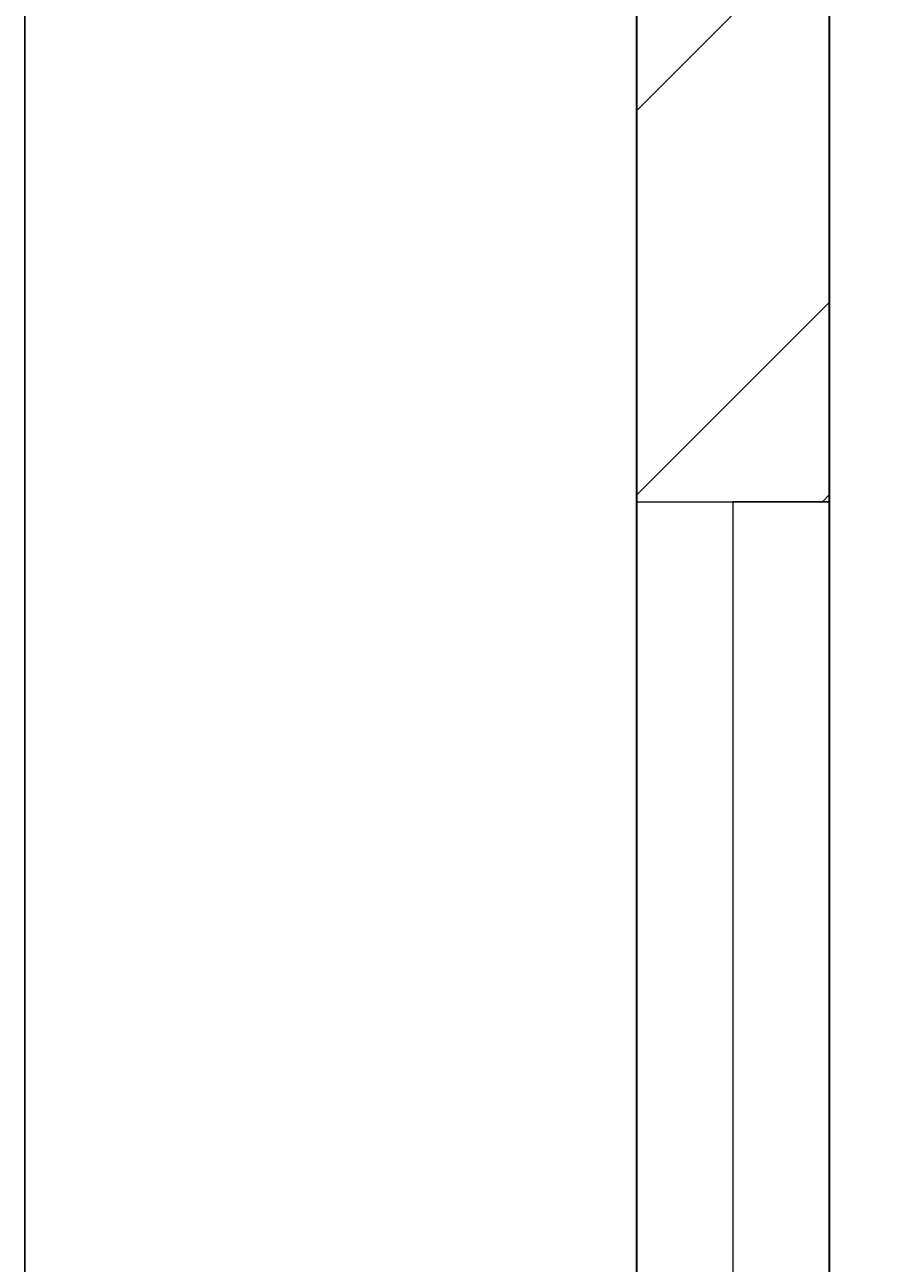
# Model space of a CAD drawing. Units: inches. Extents: x 1962 to 2771, y 1245 to 2660.
# Tile 47 of 114: x 2072 to 2092, y 2122 to 2151. Entities that reach past the tile are written whole.
import ezdxf

# ---------------------------------------------------------------- set-up
doc = ezdxf.new("R2010")
doc.units = ezdxf.units.IN
for name, color, linetype, lineweight in [('A-ANNO-DIMS', 2, 'Continuous', 18), ('A-GLAZ', 4, 'Continuous', 18), ('A-WALL', 7, 'Continuous', 35), ('A-WALL-PATT', 252, 'Continuous', 13)]:
    doc.layers.add(name, color=color, linetype=linetype, lineweight=lineweight)
doc.styles.get("Standard").update_dxf_attribs({"font": 'arial.ttf'})
doc.dimstyles.get("Standard").update_dxf_attribs({"dimtxt": 0.18, "dimasz": 0.18, "dimexe": 0.18, "dimexo": 0.0625, "dimgap": 0.09, "dimtad": 0, "dimtih": 1, "dimtoh": 1, "dimdec": 4, "dimzin": 0, "dimdsep": 46, "dimtxsty": 'Standard', "dimcen": 0.09, "dimadec": 0, "dimazin": 0, "dimtfac": 1, "dimtdec": 4, "dimtofl": 0, "dimtmove": 0, "dimatfit": 3, "dimfxl": 1, "dimtolj": 1, "dimtzin": 0, "dimarcsym": 0})

# ---------------------------------------------------------------- blocks, each defined once
blk = doc.blocks.new('WIN-60IN-A')
for p, q in [((0, 60), (4.5, 60)), ((4.5, 60), (2.25, 60)), ((2.25, 60), (2.25, 0))]:
    blk.add_line(p, q)
blk = doc.blocks.new('*D40')
at = {"layer": 'A-ANNO-DIMS', "color": 0, "lineweight": -2, "transparency": 16777216}
for p, q in [((2072.02, 2033.906), (2072.02, 2583.474)), ((2072.2, 2583.294), (2366.02, 2583.294)), ((2660.627, 2583.294), (2366.808, 2583.294)), ((2660.807, 2524.406), (2660.807, 2583.474))]:
    blk.add_line(p, q, dxfattribs=at)
at = {"layer": 'A-ANNO-DIMS', "color": 0, "transparency": 16777216}
for points in [[(2072.2, 2583.324), (2072.2, 2583.264), (2072.02, 2583.294)], [(2660.627, 2583.324), (2660.627, 2583.264), (2660.807, 2583.294)]]:
    blk.add_solid(points, dxfattribs=at)
at = {"layer": 'Defpoints', "color": 0, "transparency": 16777216}
for p in [(2660.807, 2583.294), (2660.807, 2524.344), (2072.02, 2033.844)]:
    blk.add_point(p, dxfattribs=at)
at = {"layer": 'A-ANNO-DIMS', "color": 0, "transparency": 16777216, "insert": (2366.414, 2583.294), "char_height": 0.18, "attachment_point": 5}
blk.add_mtext('\\A1;588.8', dxfattribs=at)
blk = doc.blocks.new('*D43')
at = {"layer": 'A-ANNO-DIMS', "color": 0, "lineweight": -2, "transparency": 16777216}
for p, q in [((2086.245, 2524.344), (2012.89, 2524.344)), ((2013.07, 2524.164), (2013.07, 2279.276)), ((2013.07, 2034.024), (2013.07, 2278.912)), ((2071.958, 2033.844), (2012.89, 2033.844))]:
    blk.add_line(p, q, dxfattribs=at)
at = {"layer": 'A-ANNO-DIMS', "color": 0, "transparency": 16777216}
for points in [[(2013.04, 2524.164), (2013.1, 2524.164), (2013.07, 2524.344)], [(2013.04, 2034.024), (2013.1, 2034.024), (2013.07, 2033.844)]]:
    blk.add_solid(points, dxfattribs=at)
at = {"layer": 'Defpoints', "color": 0, "transparency": 16777216}
for p in [(2086.307, 2524.344), (2013.07, 2033.844), (2072.02, 2033.844)]:
    blk.add_point(p, dxfattribs=at)
at = {"layer": 'A-ANNO-DIMS', "color": 0, "transparency": 16777216, "insert": (2013.07, 2279.094), "char_height": 0.18, "attachment_point": 5}
blk.add_mtext('\\A1;490.5', dxfattribs=at)

msp = doc.modelspace()

# ---------------------------------------------------------------- hatches: boundary and pattern name
at = {"layer": 'A-WALL-PATT'}
h = msp.add_hatch(dxfattribs=at)
h.set_pattern_fill('ANSI32', color=256)
h.paths.add_polyline_path([(2090.8074, 2467.3437), (2141.6481, 2467.3437), (2141.6481, 2469.5937), (2141.6481, 2471.8437), (2086.3074, 2471.8437), (2086.3074, 2422.5333), (2090.8074, 2422.5333)])
h.paths.add_polyline_path([(2282.7664, 2471.8437), (2204.8982, 2471.8437), (2204.8982, 2467.3437), (2234.8074, 2467.3437), (2234.8074, 2311.3437), (2228.7492, 2311.3437), (2228.7492, 2306.8437), (2234.8074, 2306.8437), (2331.9227, 2306.8437), (2331.9227, 2309.0937), (2331.9227, 2311.3437), (2239.3074, 2311.3437), (2239.3074, 2467.3437), (2282.7664, 2467.3437), (2282.7664, 2469.5937)])
h.paths.add_polyline_path([(2471.4531, 2519.8437), (2552.011, 2519.8437), (2564.3996, 2519.8437), (2564.3996, 2511.1389), (2568.8996, 2511.1389), (2568.8996, 2524.3437), (2466.9531, 2524.3437), (2466.9531, 2471.8437), (2450.0749, 2471.8437), (2446.4672, 2471.8437), (2446.4672, 2467.3437), (2450.0749, 2467.3437), (2475.9988, 2467.3437), (2475.9988, 2469.5937), (2475.9988, 2471.8437), (2471.4531, 2471.8437)])
h.paths.add_polyline_path([(2575.2231, 2469.5937), (2575.2231, 2471.8437), (2568.8996, 2471.8437), (2568.8996, 2487.1389), (2564.3996, 2487.1389), (2564.3996, 2471.8437), (2556.511, 2471.8437), (2499.2904, 2471.8437), (2499.2904, 2467.3437), (2507.8074, 2467.3437), (2507.8074, 2311.3437), (2414.863, 2311.3437), (2414.863, 2306.8437), (2512.3074, 2306.8437), (2517.0114, 2306.8437), (2517.0114, 2309.0937), (2517.0114, 2311.3437), (2512.3074, 2311.3437), (2512.3074, 2467.3437), (2575.2231, 2467.3437)])
h.paths.add_polyline_path([(2660.8074, 2471.8437), (2600.9602, 2471.8437), (2600.9602, 2467.3437), (2656.3074, 2467.3437), (2656.3074, 2432.5704), (2660.8074, 2432.5704)])
h.paths.add_polyline_path([(2660.8074, 2372.5704), (2656.3074, 2372.5704), (2656.3074, 2311.3437), (2600.276, 2311.3437), (2600.276, 2309.0937), (2600.276, 2306.8437), (2656.3074, 2306.8437), (2656.3074, 2296.2593), (2660.8074, 2296.2593)])
h.paths.add_polyline_path([(2572.3074, 2306.8437), (2577.1385, 2306.8437), (2577.1385, 2311.3437), (2551.082, 2311.3437), (2551.082, 2306.8437), (2567.8074, 2306.8437), (2567.8074, 2258.8437), (2540.0574, 2258.8437), (2540.0574, 2256.5937), (2540.0574, 2254.3437), (2567.8074, 2254.3437), (2656.3074, 2254.3437), (2656.3074, 2236.9085), (2660.8074, 2236.9085), (2660.8074, 2272.2593), (2656.3074, 2272.2593), (2656.3074, 2258.8437), (2572.3074, 2258.8437)])
h.paths.add_polyline_path([(2512.3074, 2254.3437), (2518.8716, 2254.3437), (2518.8716, 2256.5937), (2518.8716, 2258.8437), (2507.8074, 2258.8437), (2507.8074, 2177.8437), (2567.8074, 2177.8437), (2567.8074, 2172.9628), (2572.3074, 2172.9628), (2572.3074, 2177.8437), (2656.3074, 2177.8437), (2656.3074, 2166.4846), (2660.8074, 2166.4846), (2660.8074, 2200.9085), (2656.3074, 2200.9085), (2656.3074, 2182.3437), (2512.3074, 2182.3437)])
h.paths.add_polyline_path([(2656.3074, 2129.8437), (2572.3074, 2129.8437), (2572.3074, 2150.3044), (2570.0574, 2150.3044), (2567.8074, 2150.3044), (2567.8074, 2129.8437), (2507.8074, 2129.8437), (2507.8074, 2116.3027), (2510.0574, 2116.3027), (2512.3074, 2116.3027), (2512.3074, 2125.3437), (2567.8074, 2125.3437), (2572.3074, 2125.3437), (2656.3074, 2125.3437)])
h.paths.add_polyline_path([(2090.8074, 2362.5333), (2086.3074, 2362.5333), (2086.3074, 2298.6242), (2090.8074, 2298.6242), (2090.8074, 2306.8437), (2174.8074, 2306.8437), (2174.8074, 2286.4178), (2179.3074, 2286.4178), (2179.3074, 2306.8437), (2192.8641, 2306.8437), (2192.8641, 2309.0937), (2192.8641, 2311.3437), (2090.8074, 2311.3437)])
h.paths.add_polyline_path([(2209.156, 2258.8437), (2179.3074, 2258.8437), (2179.3074, 2263.2236), (2177.0574, 2263.2236), (2174.8074, 2263.2236), (2174.8074, 2258.8437), (2090.8074, 2258.8437), (2090.8074, 2274.6242), (2086.3074, 2274.6242), (2086.3074, 2238.2967), (2088.5574, 2238.2967), (2090.8074, 2238.2967), (2090.8074, 2254.3437), (2209.156, 2254.3437)])
h.paths.add_polyline_path([(2090.8074, 2177.8437), (2234.8074, 2177.8437), (2234.8074, 2173.1428), (2239.3074, 2173.1428), (2239.3074, 2258.8437), (2230.8442, 2258.8437), (2230.8442, 2256.5937), (2230.8442, 2254.3437), (2234.8074, 2254.3437), (2234.8074, 2182.3437), (2090.8074, 2182.3437), (2090.8074, 2202.2967), (2086.3074, 2202.2967), (2086.3074, 2140.0389), (2090.8074, 2140.0389)])
h.paths.add_polyline_path([(2090.8074, 2080.0389), (2086.3074, 2080.0389), (2086.3074, 2033.8437), (2090.8074, 2033.8437)], flags=17)
h.paths.add_polyline_path([(2244.9405, 2033.8437), (2239.3074, 2033.8437), (2239.3074, 2142.0665), (2237.2592, 2142.0665), (2234.8074, 2142.0665), (2234.8074, 2033.8437), (2090.8074, 2033.8437), (2076.5204, 2033.8437), (2072.0204, 2033.8437), (2072.0204, 2000.4493), (2076.5204, 2000.4493), (2076.5204, 2029.3437), (2090.8074, 2029.3437), (2244.9405, 2029.3437), (2244.9405, 2031.5937)])
h.paths.add_polyline_path([(2234.8074, 1933.3437), (2076.5204, 1933.3437), (2076.5204, 1952.4493), (2074.2704, 1952.4493), (2072.0204, 1952.4493), (2072.0204, 1933.3437), (2072.0204, 1928.8437), (2234.8074, 1928.8437)])
h.paths.add_polyline_path([(2090.8074, 1928.8437), (2086.3074, 1928.8437), (2086.3074, 1906.5013), (2090.8074, 1906.5013)])
h.paths.add_polyline_path([(2090.8074, 1846.5013), (2086.3074, 1846.5013), (2086.3074, 1769.9917), (2088.5574, 1769.9917), (2090.8074, 1769.9917), (2090.8074, 1780.3437), (2234.8074, 1780.3437), (2234.8074, 1708.3437), (2230.3764, 1708.3437), (2230.3764, 1703.8437), (2239.3074, 1703.8437), (2239.3074, 1792.6669), (2237.0574, 1792.6669), (2234.8074, 1792.6669), (2234.8074, 1784.8437), (2090.8074, 1784.8437)])
h.paths.add_polyline_path([(2239.3074, 1928.8437), (2244.9405, 1928.8437), (2244.9405, 1931.0937), (2244.9405, 1933.3437), (2234.8074, 1933.3437), (2234.8074, 1928.8437), (2234.8074, 1825.5949), (2239.3074, 1825.5949)])
h.paths.add_polyline_path([(2148.0425, 1649.0937), (2148.0425, 1651.3437), (2090.8074, 1651.3437), (2090.8074, 1646.8437), (2148.0425, 1646.8437)], flags=0)
h.paths.add_polyline_path([(2207.5601, 1708.3437), (2090.8074, 1708.3437), (2090.8074, 1703.8437), (2174.8074, 1703.8437), (2174.8074, 1651.3437), (2170.4457, 1651.3437), (2170.4457, 1646.8437), (2195.9924, 1646.8437), (2195.9924, 1649.0937), (2195.9924, 1651.3437), (2179.3074, 1651.3437), (2179.3074, 1703.8437), (2207.5601, 1703.8437), (2207.5601, 1706.0937)])
h.paths.add_polyline_path([(2090.8074, 1733.9917), (2086.3074, 1733.9917), (2086.3074, 1696.1032), (2088.5574, 1696.1032), (2090.8074, 1696.1032)])
h.paths.add_polyline_path([(2090.8074, 1672.1032), (2086.3074, 1672.1032), (2086.3074, 1600.3335), (2090.8074, 1600.3335)])
h.paths.add_polyline_path([(2090.8074, 1540.3335), (2086.3074, 1540.3335), (2086.3074, 1486.3437), (2139.6766, 1486.3437), (2139.6766, 1490.8437), (2090.8074, 1490.8437)])
h.paths.add_polyline_path([(2302.3876, 1490.8437), (2239.3074, 1490.8437), (2239.3074, 1646.8437), (2335.9994, 1646.8437), (2335.9994, 1651.3437), (2229.884, 1651.3437), (2229.884, 1646.8437), (2234.8074, 1646.8437), (2234.8074, 1490.8437), (2202.7103, 1490.8437), (2202.7103, 1488.5937), (2202.7103, 1486.3437), (2275.0699, 1486.3437), (2275.0699, 1475.772), (2279.5699, 1475.772), (2279.5699, 1486.3437), (2302.3876, 1486.3437)])
h.paths.add_polyline_path([(2279.5699, 1451.772), (2275.0699, 1451.772), (2275.0699, 1438.3437), (2174.8074, 1438.3437), (2174.8074, 1486.3437), (2179.7922, 1486.3437), (2179.7922, 1490.8437), (2163.3585, 1490.8437), (2163.3585, 1488.5937), (2163.3585, 1486.3437), (2170.3074, 1486.3437), (2170.3074, 1433.8437), (2279.5699, 1433.8437)])
h.paths.add_polyline_path([(2427.2363, 1490.8437), (2375.8074, 1490.8437), (2375.8074, 1646.8437), (2381.6401, 1646.8437), (2381.6401, 1651.3437), (2365.887, 1651.3437), (2365.887, 1649.0937), (2365.887, 1646.8437), (2371.3074, 1646.8437), (2371.3074, 1490.8437), (2327.5627, 1490.8437), (2327.5627, 1488.5937), (2327.5627, 1486.3437), (2371.3074, 1486.3437), (2371.3074, 1433.8437), (2375.8074, 1433.8437), (2375.8074, 1486.3437), (2427.2363, 1486.3437)])
h.paths.add_polyline_path([(2512.3074, 1646.8437), (2519.4351, 1646.8437), (2519.4351, 1649.0937), (2519.4351, 1651.3437), (2507.8074, 1651.3437), (2416.0063, 1651.3437), (2416.0063, 1649.0937), (2416.0063, 1646.8437), (2507.8074, 1646.8437), (2507.8074, 1490.8437), (2497.0532, 1490.8437), (2497.0532, 1488.5937), (2497.0532, 1486.3437), (2574.9344, 1486.3437), (2574.9344, 1476.0181), (2579.4344, 1476.0181), (2579.4344, 1486.3437), (2584.4872, 1486.3437), (2584.3074, 1490.8437), (2512.3074, 1490.8437)])
h.paths.add_polyline_path([(2470.5091, 1486.3437), (2473.9767, 1486.3437), (2473.9767, 1490.8437), (2449.6605, 1490.8437), (2449.6605, 1488.5937), (2449.6605, 1486.3437), (2466.0091, 1486.3437), (2466.0091, 1433.8437), (2470.5091, 1433.8437), (2579.4344, 1433.8437), (2579.4344, 1452.0181), (2574.9344, 1452.0181), (2574.9344, 1438.3437), (2554.5091, 1438.3437), (2470.5091, 1438.3437)])
h.paths.add_polyline_path([(2656.3074, 1490.8437), (2611.86, 1490.8437), (2611.86, 1486.3437), (2656.3074, 1486.3437)])
h.paths.add_polyline_path([(2660.8074, 1532.7007), (2658.5574, 1532.7007), (2656.3074, 1532.7007), (2656.3074, 1486.3437), (2660.8074, 1486.3437)])
h.paths.add_polyline_path([(2660.8074, 1664.9663), (2656.3074, 1664.9663), (2656.3074, 1651.3437), (2602.2313, 1651.3437), (2602.2313, 1646.8437), (2656.3074, 1646.8437), (2656.3074, 1592.7007), (2660.8074, 1592.7007)])
h.paths.add_polyline_path([(2660.8074, 1724.5221), (2656.3074, 1724.5221), (2656.3074, 1703.8437), (2542.4725, 1703.8437), (2542.4725, 1699.3437), (2567.8074, 1699.3437), (2567.8074, 1651.3437), (2552.7766, 1651.3437), (2552.7766, 1649.0937), (2552.7766, 1646.8437), (2577.2878, 1646.8437), (2577.2878, 1649.0937), (2577.2878, 1651.3437), (2572.3074, 1651.3437), (2572.3074, 1699.3437), (2656.3074, 1699.3437), (2656.3074, 1688.9663), (2660.8074, 1688.9663)])
h.paths.add_polyline_path([(2660.8074, 1880.6524), (2656.3074, 1880.6524), (2656.3074, 1832.8437), (2512.3074, 1832.8437), (2512.3074, 1837.8959), (2507.8074, 1837.8959), (2507.8074, 1828.3437), (2567.8074, 1828.3437), (2567.8074, 1804.3437), (2572.3074, 1804.3437), (2572.3074, 1828.3437), (2656.3074, 1828.3437), (2656.3074, 1818.6778), (2660.8074, 1818.6778)])
h.paths.add_polyline_path([(2660.8074, 1794.6778), (2656.3074, 1794.6778), (2656.3074, 1780.3437), (2572.3074, 1780.3437), (2572.3074, 1783.0303), (2570.0574, 1783.0303), (2567.8074, 1783.0303), (2567.8074, 1780.3437), (2507.8074, 1780.3437), (2507.8074, 1699.3437), (2517.8858, 1699.3437), (2517.8858, 1701.5937), (2517.8858, 1703.8437), (2512.3074, 1703.8437), (2512.3074, 1775.8437), (2656.3074, 1775.8437), (2656.3074, 1760.5221), (2660.8074, 1760.5221)])
h.paths.add_polyline_path([(2660.8074, 1981.3437), (2660.8074, 2020.2808), (2658.5574, 2020.2808), (2656.3074, 2020.2808), (2656.3074, 1981.3437), (2512.3074, 1981.3437), (2512.3074, 2086.6996), (2507.8074, 2086.6996), (2507.8074, 1981.3437), (2375.8074, 1981.3437), (2375.8074, 1986.8505), (2373.5574, 1986.8505), (2371.3074, 1986.8505), (2371.3074, 1973.2607), (2375.8074, 1973.2607), (2375.8074, 1976.8437), (2507.8074, 1976.8437), (2507.8074, 1865.4281), (2510.0574, 1865.4281), (2512.3074, 1865.4281), (2512.3074, 1976.8437), (2660.8074, 1976.8437)])
h.paths.add_polyline_path([(2375.8074, 1940.297), (2373.5574, 1940.297), (2371.3074, 1940.297), (2371.3074, 1933.3437), (2278.4434, 1933.3437), (2278.4434, 1928.8437), (2371.3074, 1928.8437), (2371.3074, 1651.3437), (2375.8074, 1651.3437)])
h.paths.add_polyline_path([(2660.8074, 1976.8437), (2656.3074, 1976.8437), (2656.3074, 1940.6524), (2660.8074, 1940.6524)], flags=17)
h.paths.add_polyline_path([(2660.8074, 2142.4846), (2656.3074, 2142.4846), (2656.3074, 2080.2808), (2660.8074, 2080.2808)])
h.paths.add_polyline_path([(2381.4189, 2311.3437), (2375.8074, 2311.3437), (2375.8074, 2467.3437), (2424.7242, 2467.3437), (2424.7242, 2469.5937), (2424.7242, 2471.8437), (2375.8074, 2471.8437), (2375.8074, 2524.3437), (2371.3074, 2524.3437), (2371.3074, 2471.8437), (2307.2097, 2471.8437), (2307.2097, 2467.3437), (2371.3074, 2467.3437), (2371.3074, 2311.3437), (2366.8901, 2311.3437), (2366.8901, 2306.8437), (2371.3074, 2306.8437), (2371.3074, 2033.8437), (2279.6589, 2033.8437), (2279.6589, 2029.3437), (2371.3074, 2029.3437), (2371.3074, 2014.2598), (2375.8074, 2014.2598), (2375.8074, 2306.8437), (2381.4189, 2306.8437)])
h.paths.add_polyline_path([(2263.3074, 2524.3437), (2170.3074, 2524.3437), (2170.3074, 2519.8437), (2170.3074, 2471.8437), (2165.0312, 2471.8437), (2165.0312, 2467.3437), (2179.6721, 2467.3437), (2179.6721, 2469.5161), (2179.6721, 2471.8437), (2174.8074, 2471.8437), (2174.8074, 2519.8437), (2258.8074, 2519.8437), (2258.8074, 2511.6436), (2263.3074, 2511.6436)])
h.paths.add_polyline_path([(2245.0232, 1361.4123), (2492.9468, 1361.4123), (2492.9468, 1398.505), (2245.0232, 1398.505)], flags=9)
h.paths.add_polyline_path([(2388.1434, 2086.6936), (2425.0704, 2086.6936), (2425.0704, 2105.3509), (2388.1434, 2105.3509)], flags=9)
h.paths.add_polyline_path([(2404.922, 2242.6744), (2445.7337, 2242.6744), (2445.7337, 2261.3318), (2404.922, 2261.3318)], flags=9)
h.paths.add_polyline_path([(2269.4107, 2156.7935), (2306.3378, 2156.7935), (2306.3378, 2175.4508), (2269.4107, 2175.4508)], flags=9)
h.paths.add_polyline_path([(2269.3277, 2233.4343), (2306.2547, 2233.4343), (2306.2547, 2252.0917), (2269.3277, 2252.0917)], flags=9)
h.paths.add_polyline_path([(2431.6052, 2320.6922), (2470.4456, 2320.6922), (2470.4456, 2339.3495), (2431.6052, 2339.3495)], flags=25)
h.paths.add_polyline_path([(2249.6902, 2315.7608), (2288.5306, 2315.7608), (2288.5306, 2334.4182), (2249.6902, 2334.4182)], flags=25)
h.paths.add_polyline_path([(2096.9301, 2314.3181), (2135.7704, 2314.3181), (2135.7704, 2332.9755), (2096.9301, 2332.9755)], flags=25)
h.paths.add_polyline_path([(2134.3475, 2285.7089), (2161.4655, 2285.7089), (2161.4655, 2304.3662), (2134.3475, 2304.3662)], flags=9)
h.paths.add_polyline_path([(2126.5155, 2209.4076), (2159.9227, 2209.4076), (2159.9227, 2228.065), (2126.5155, 2228.065)], flags=25)
h.paths.add_polyline_path([(2110.5753, 2141.5299), (2149.4157, 2141.5299), (2149.4157, 2160.1872), (2110.5753, 2160.1872)], flags=25)
h.paths.add_polyline_path([(2249.8618, 1968.3317), (2286.3966, 1968.3317), (2286.3966, 1986.989), (2249.8618, 1986.989)], flags=9)
h.paths.add_polyline_path([(2395.9507, 1777.0051), (2436.7624, 1777.0051), (2436.7624, 1795.6625), (2395.9507, 1795.6625)], flags=9)
h.paths.add_polyline_path([(2398.5259, 1888.5651), (2435.0062, 1888.5651), (2435.0062, 1907.2224), (2398.5259, 1907.2224)], flags=25)
h.paths.add_polyline_path([(2259.3506, 1728.3559), (2296.2776, 1728.3559), (2296.2776, 1747.0132), (2259.3506, 1747.0132)], flags=9)
h.paths.add_polyline_path([(2271.3698, 1845.268), (2308.2968, 1845.268), (2308.2968, 1863.9253), (2271.3698, 1863.9253)], flags=9)
h.paths.add_polyline_path([(2120.9355, 1786.3027), (2159.7759, 1786.3027), (2159.7759, 1804.9601), (2120.9355, 1804.9601)], flags=25)
h.paths.add_polyline_path([(2121.3164, 1732.1043), (2154.7236, 1732.1043), (2154.7236, 1750.7616), (2121.3164, 1750.7616)], flags=25)
h.paths.add_polyline_path([(2118.3706, 1678.8997), (2147.5282, 1678.8997), (2147.5282, 1697.557), (2118.3706, 1697.557)], flags=25)
h.paths.add_polyline_path([(2385.9227, 1493.557), (2424.763, 1493.557), (2424.763, 1512.2143), (2385.9227, 1512.2143)], flags=25)
h.paths.add_polyline_path([(2248.7058, 1500.0256), (2287.5462, 1500.0256), (2287.5462, 1518.6829), (2248.7058, 1518.6829)], flags=25)
h.paths.add_polyline_path([(2104.1669, 1617.3771), (2143.0073, 1617.3771), (2143.0073, 1636.0344), (2104.1669, 1636.0344)], flags=9)
h.paths.add_polyline_path([(2096.0714, 1447.8824), (2137.3845, 1447.8824), (2137.3845, 1458.1859), (2096.0714, 1458.1859)], flags=9)
h.paths.add_polyline_path([(2180.6114, 1440.325), (2209.7689, 1440.325), (2209.7689, 1458.9823), (2180.6114, 1458.9823)], flags=25)
h.paths.add_polyline_path([(2316.1698, 1447.9637), (2357.4829, 1447.9637), (2357.4829, 1458.2673), (2316.1698, 1458.2673)], flags=9)
h.paths.add_polyline_path([(2397.6187, 1447.9637), (2438.9318, 1447.9637), (2438.9318, 1458.2673), (2397.6187, 1458.2673)], flags=9)
h.paths.add_polyline_path([(2473.0778, 1439.5953), (2502.2354, 1439.5953), (2502.2354, 1458.2527), (2473.0778, 1458.2527)], flags=25)
h.paths.add_polyline_path([(2589.7027, 1447.8819), (2631.0158, 1447.8819), (2631.0158, 1458.1855), (2589.7027, 1458.1855)], flags=9)
h.paths.add_polyline_path([(2522.4009, 1497.5285), (2561.2413, 1497.5285), (2561.2413, 1516.1859), (2522.4009, 1516.1859)], flags=25)
h.paths.add_polyline_path([(2579.6565, 1671.3482), (2608.8141, 1671.3482), (2608.8141, 1690.0056), (2579.6565, 1690.0056)], flags=25)
h.paths.add_polyline_path([(2544.7038, 1725.5064), (2578.1111, 1725.5064), (2578.1111, 1744.1637), (2544.7038, 1744.1637)], flags=25)
h.paths.add_polyline_path([(2578.1191, 1807.472), (2607.2766, 1807.472), (2607.2766, 1826.1293), (2578.1191, 1826.1293)], flags=25)
h.paths.add_polyline_path([(2595.0614, 1835.1839), (2633.9018, 1835.1839), (2633.9018, 1853.8413), (2595.0614, 1853.8413)], flags=25)
h.paths.add_polyline_path([(2567.0097, 2097.7035), (2605.8501, 2097.7035), (2605.8501, 2116.3609), (2567.0097, 2116.3609)], flags=9)
h.paths.add_polyline_path([(2586.644, 2134.6454), (2615.8015, 2134.6454), (2615.8015, 2153.3027), (2586.644, 2153.3027)], flags=9)
h.paths.add_polyline_path([(2544.6185, 2212.6783), (2578.0258, 2212.6783), (2578.0258, 2231.3356), (2544.6185, 2231.3356)], flags=25)
h.paths.add_polyline_path([(2577.0273, 2256.9023), (2606.1849, 2256.9023), (2606.1849, 2275.5597), (2577.0273, 2275.5597)], flags=24)
h.paths.add_polyline_path([(2605.2683, 2315.2821), (2644.1087, 2315.2821), (2644.1087, 2333.9395), (2605.2683, 2333.9395)], flags=25)
h.paths.add_polyline_path([(2583.1244, 2496.1815), (2624.4375, 2496.1815), (2624.4375, 2506.4851), (2583.1244, 2506.4851)], flags=9)
h.paths.add_polyline_path([(2474.761, 2497.0823), (2503.9185, 2497.0823), (2503.9185, 2515.7397), (2474.761, 2515.7397)], flags=25)
h.paths.add_polyline_path([(2387.5787, 2494.2563), (2428.902, 2494.2563), (2428.902, 2504.5598), (2387.5787, 2504.5598)], flags=9)
h.paths.add_polyline_path([(2300.1657, 2500.1564), (2341.4788, 2500.1564), (2341.4788, 2510.46), (2300.1657, 2510.46)], flags=25)
h.paths.add_polyline_path([(2176.8589, 2497.5843), (2206.0165, 2497.5843), (2206.0165, 2516.2416), (2176.8589, 2516.2416)], flags=25)
h.paths.add_polyline_path([(2097.4668, 2494.9762), (2138.7799, 2494.9762), (2138.7799, 2505.2798), (2097.4668, 2505.2798)], flags=9)

# ---------------------------------------------------------------- linework, layer by layer
at = {"layer": 'A-WALL'}
for p, q in [((2086.3074, 2471.8437), (2086.3074, 2033.8437)), ((2090.8074, 2177.8437), (2090.8074, 2033.8437))]:
    msp.add_line(p, q, dxfattribs=at)

# ---------------------------------------------------------------- block references
at = {"layer": 'A-GLAZ'}
msp.add_blockref('WIN-60IN-A', (2086.3074, 2080.0389), dxfattribs=at)

# ---------------------------------------------------------------- dimensions: what is measured, and where the dimension line sits
at = {"layer": 'A-ANNO-DIMS'}
dim = msp.add_linear_dim(base=(2660.8074, 2583.2937), p1=(2072.0204, 2033.8437), p2=(2660.8074, 2524.3437), dimstyle='Standard', override={"dimdec": 1, "dimlfac": 1, "dimrnd": 0, "dimzin": 0, "dimdsep": 46, "dimlunit": 2}, dxfattribs=at)
dim.commit()
dim.dimension.update_dxf_attribs({"geometry": '*D40', "text_midpoint": (2366.4139, 2583.2937)})
dim = msp.add_linear_dim(base=(2013.0704, 2033.8437), p1=(2086.3074, 2524.3437), p2=(2072.0204, 2033.8437), angle=90, dimstyle='Standard', override={"dimdec": 1, "dimlfac": 1, "dimrnd": 0, "dimzin": 0, "dimdsep": 46, "dimlunit": 2}, dxfattribs=at)
dim.commit()
dim.dimension.update_dxf_attribs({"geometry": '*D43', "text_midpoint": (2013.0704, 2279.0937)})

doc.saveas('drawing.dxf')
